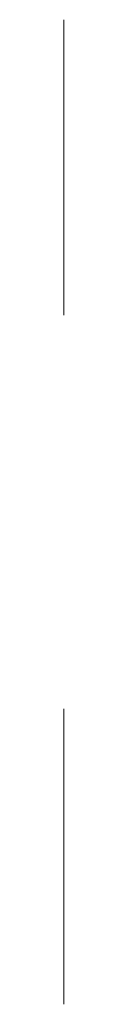
# Model space of a CAD drawing. Units: millimetres. Extents: x 474.4 to 474.4, y 226.5 to 266.5.
import ezdxf

# ---------------------------------------------------------------- set-up
doc = ezdxf.new("R2010")
doc.units = ezdxf.units.MM
doc.layers.add('M-CONS', color=8, linetype='Continuous', lineweight=13)

msp = doc.modelspace()

# ---------------------------------------------------------------- linework, layer by layer
at = {"layer": 'M-CONS', "extrusion": (1, 0, 0)}
msp.add_line((474.392, 266.508, 228.634), (474.392, 254.508, 228.634), dxfattribs=at)
at = {"layer": 'M-CONS'}
msp.add_line((474.392, 238.508, 228.634), (474.392, 226.508, 228.634), dxfattribs=at)

doc.saveas('drawing.dxf')
